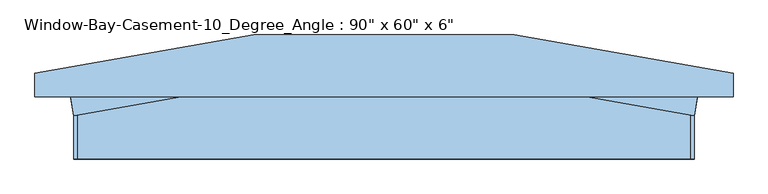
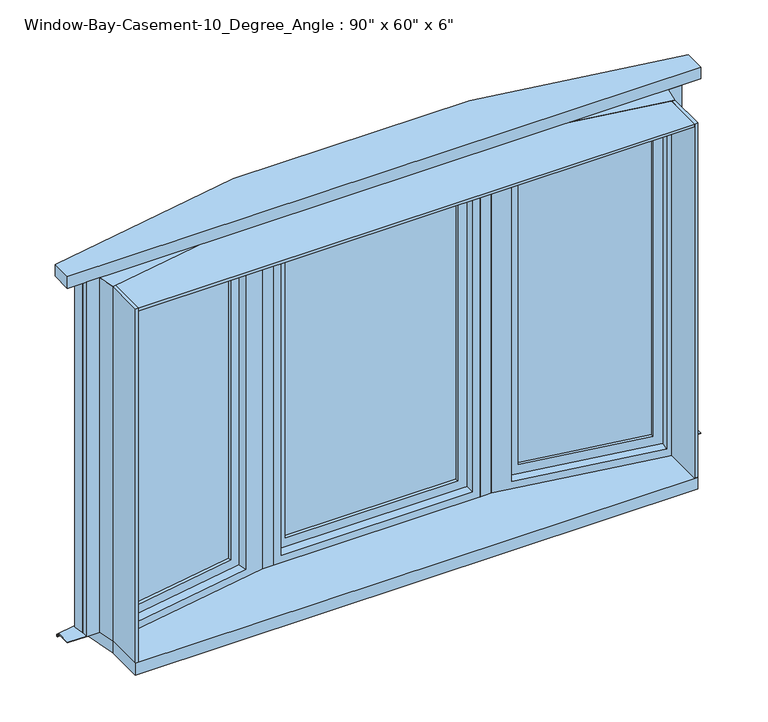
"""IFC4 building model written with IfcOpenShell, lengths in millimetres: window geometry."""

from ifc_helpers import new_model, si_unit, frame, origin, place, context, project, spatial, polyline, outline, extrude, faceted_brep, source, transform, mapped, element, save


def window_bf21e6cb(model_context):
    return source(origin(), model_context, "Body", "SolidModel", [
        extrude(outline(polyline([(1086.3405037, 126.4293252), (1085.2378377, 120.175796), (588.6035631, 207.7458181), (589.7062291, 213.9993474), (1086.3405037, 126.4293252)])), frame((0.0, 0.0, 730.25), z_axis=(0.0, 0.0, 1.0), x_axis=(1.0, 0.0, 0.0)), (0.0, 0.0, 1.0), 1384.3),
        extrude(outline(polyline([(1084.1351718, 113.9222667), (1083.0325059, 107.6687375), (586.3982313, 195.2387597), (587.5008972, 201.4922889), (1084.1351718, 113.9222667)])), frame((0.0, 0.0, 730.25), z_axis=(0.0, 0.0, 1.0), x_axis=(1.0, 0.0, 0.0)), (0.0, 0.0, 1.0), 1384.3),
        extrude(outline(polyline([(1441.45, 57.15), (1441.45, -561.4456588), (-57.15, -561.4456588), (-57.15, 57.15), (1441.45, 57.15)]), holes=[polyline([(1384.3, -504.2956588), (1384.3, 0.0), (0.0, 0.0), (0.0, -504.2956588), (1384.3, -504.2956588)])]), frame((1080.827174, 95.1616791, 730.25), z_axis=(0.17364817766693028, 0.9848077530122081, 0.0), x_axis=(0.0, 0.0, 1.0)), (0.0, 0.0, 1.0), 44.45),
        faceted_brep([(464.7780905, 165.1, 2184.4), (1143.0, 45.5111785, 2184.4), (1155.1293252, 114.3, 2184.4), (1210.6708887, 114.3, 2184.4), (1210.6708887, 136.7463187, 2184.4), (473.6669387, 266.7, 2184.4), (1137.1089371, 85.2376857, 2171.7), (527.9111363, 192.6556946, 2171.7), (538.9377956, 255.1909869, 2171.7), (1148.1355964, 147.772978, 2171.7), (1111.7323538, 51.0245081, 2152.65), (540.0557285, 151.8265214, 2152.65), (546.671724, 189.3476968, 2152.65), (1118.3483494, 88.5456835, 2152.65), (527.9111363, 192.6556946, 673.1), (538.9377956, 255.1909869, 673.1), (540.0557285, 151.8265214, 692.15), (546.671724, 189.3476968, 692.15), (473.6669387, 266.7, 660.4), (1210.6708887, 136.7463187, 660.4), (1210.6708887, 114.3, 660.4), (1155.1293252, 114.3, 660.4), (1143.0, 45.5111785, 660.4), (464.7780905, 165.1, 660.4), (1137.1089371, 85.2376857, 673.1), (1148.1355964, 147.772978, 673.1), (1111.7323538, 51.0245081, 692.15), (1118.3483494, 88.5456835, 692.15)], [[[0, 1, 2, 3, 4, 5]], [[6, 7, 8, 9]], [[10, 11, 12, 13]], [[7, 14, 15, 8]], [[11, 16, 17, 12]], [[18, 19, 20, 21, 22, 23]], [[14, 24, 25, 15]], [[16, 26, 27, 17]], [[22, 21, 2, 1]], [[4, 19, 18, 5], [8, 15, 25, 9]], [[9, 25, 24, 6]], [[6, 24, 14, 7], [12, 17, 27, 13]], [[13, 27, 26, 10]], [[1, 0, 23, 22], [10, 26, 16, 11]], [[5, 18, 23, 0]], [[2, 21, 20, 3]], [[3, 20, 19, 4]]]),
        extrude(outline(polyline([(-1086.3405037, 126.4293252), (-589.7062291, 213.9993474), (-588.6035631, 207.7458181), (-1085.2378377, 120.175796), (-1086.3405037, 126.4293252)])), frame((0.0, 0.0, 730.25), z_axis=(0.0, 0.0, 1.0), x_axis=(1.0, 0.0, 0.0)), (0.0, 0.0, 1.0), 1384.3),
        extrude(outline(polyline([(-1084.1351718, 113.9222667), (-587.5008972, 201.4922889), (-586.3982313, 195.2387597), (-1083.0325059, 107.6687375), (-1084.1351718, 113.9222667)])), frame((0.0, 0.0, 730.25), z_axis=(0.0, 0.0, 1.0), x_axis=(1.0, 0.0, 0.0)), (0.0, 0.0, 1.0), 1384.3),
        extrude(outline(polyline([(1441.45, -57.15), (-57.15, -57.15), (-57.15, 561.4456588), (1441.45, 561.4456588), (1441.45, -57.15)]), holes=[polyline([(1384.3, 504.2956588), (0.0, 504.2956588), (0.0, 0.0), (1384.3, 0.0), (1384.3, 504.2956588)])]), frame((-1080.827174, 95.1616791, 730.25), z_axis=(-0.17364817766693028, 0.9848077530122081, 0.0), x_axis=(0.0, 0.0, 1.0)), (0.0, 0.0, 1.0), 44.45),
        faceted_brep([(-464.7780905, 165.1, 2184.4), (-473.6669387, 266.7, 2184.4), (-1210.6708887, 136.7463187, 2184.4), (-1210.6708887, 114.3, 2184.4), (-1155.1293252, 114.3, 2184.4), (-1143.0, 45.5111785, 2184.4), (-1137.1089371, 85.2376857, 2171.7), (-1148.1355964, 147.772978, 2171.7), (-538.9377956, 255.1909869, 2171.7), (-527.9111363, 192.6556946, 2171.7), (-1111.7323538, 51.0245081, 2152.65), (-1118.3483494, 88.5456835, 2152.65), (-546.671724, 189.3476968, 2152.65), (-540.0557285, 151.8265214, 2152.65), (-538.9377956, 255.1909869, 673.1), (-527.9111363, 192.6556946, 673.1), (-546.671724, 189.3476968, 692.15), (-540.0557285, 151.8265214, 692.15), (-473.6669387, 266.7, 660.4), (-464.7780905, 165.1, 660.4), (-1143.0, 45.5111785, 660.4), (-1155.1293252, 114.3, 660.4), (-1210.6708887, 114.3, 660.4), (-1210.6708887, 136.7463187, 660.4), (-1148.1355964, 147.772978, 673.1), (-1137.1089371, 85.2376857, 673.1), (-1118.3483494, 88.5456835, 692.15), (-1111.7323538, 51.0245081, 692.15)], [[[0, 1, 2, 3, 4, 5]], [[6, 7, 8, 9]], [[10, 11, 12, 13]], [[9, 8, 14, 15]], [[13, 12, 16, 17]], [[18, 19, 20, 21, 22, 23]], [[15, 14, 24, 25]], [[17, 16, 26, 27]], [[20, 5, 4, 21]], [[2, 1, 18, 23], [8, 7, 24, 14]], [[7, 6, 25, 24]], [[6, 9, 15, 25], [12, 11, 26, 16]], [[11, 10, 27, 26]], [[5, 20, 19, 0], [10, 13, 17, 27]], [[1, 0, 19, 18]], [[4, 3, 22, 21]], [[3, 2, 23, 22]]]),
        faceted_brep([(-478.1113628, 317.5, 660.4), (-478.1113628, 317.5, 653.0697935), (478.1113628, 317.5, 653.0697935), (478.1113628, 317.5, 660.4), (-473.6669387, 266.7, 663.1486341), (-473.6669387, 266.7, 660.4), (473.6669387, 266.7, 660.4), (473.6669387, 266.7, 663.1486341), (-478.2335845, 318.897, 654.4483503), (-478.2335845, 318.897, 663.1486341), (478.2335845, 318.897, 663.1486341), (478.2335845, 318.897, 654.4483503), (479.3446905, 331.597, 652.2089977), (-479.3446905, 331.597, 652.2089977), (479.3446905, 331.597, 643.2668038), (-479.3446905, 331.597, 643.2668038), (-478.9980255, 327.6346, 644.7270038), (-478.9980255, 327.6346, 643.2668038), (478.9980255, 327.6346, 643.2668038), (478.9980255, 327.6346, 644.7270038), (-479.2046912, 329.9968, 650.8662705), (-479.2046912, 329.9968, 644.7270038), (479.2046912, 329.9968, 644.7270038), (479.2046912, 329.9968, 650.8662705), (-1286.8726318, 174.8935673, 660.4), (-1286.8726318, 174.8935673, 653.0697935), (1286.8726318, 174.8935673, 660.4), (1286.8726318, 114.3, 660.4), (1210.6726318, 114.3, 660.4), (1210.6726318, 136.7460114, 660.4), (-1210.6726318, 136.7460114, 660.4), (-1210.6726318, 114.3, 660.4), (-1286.8726318, 114.3, 660.4), (-1210.6726318, 136.7460114, 663.1486341), (1210.6726318, 136.7460114, 663.1486341), (1210.6726318, 114.3, 663.1486341), (1286.8726318, 114.3, 663.1486341), (1286.8726318, 176.3121183, 663.1486341), (-1286.8726318, 176.3121183, 663.1486341), (-1286.8726318, 114.3, 663.1486341), (-1210.6726318, 114.3, 663.1486341), (-1286.8726318, 176.3121183, 654.4483503), (-1286.8726318, 189.2080363, 652.2089977), (-1286.8726318, 189.2080363, 643.2668038), (1286.8726318, 189.2080363, 643.2668038), (1286.8726318, 185.1845099, 643.2668038), (-1286.8726318, 185.1845099, 643.2668038), (-1286.8726318, 185.1845099, 644.7270038), (1286.8726318, 185.1845099, 644.7270038), (1286.8726318, 187.5831506, 644.7270038), (-1286.8726318, 187.5831506, 644.7270038), (-1286.8726318, 187.5831506, 650.8662705), (1286.8726318, 174.8935673, 653.0697935), (1286.8726318, 176.3121183, 654.4483503), (1286.8726318, 189.2080363, 652.2089977), (1286.8726318, 187.5831506, 650.8662705)], [[[0, 1, 2, 3]], [[4, 5, 6, 7]], [[8, 9, 10, 11]], [[8, 11, 12, 13]], [[13, 12, 14, 15]], [[16, 17, 18, 19]], [[20, 21, 22, 23]], [[2, 1, 20, 23]], [[1, 0, 24, 25]], [[0, 3, 26, 27, 28, 29, 6, 5, 30, 31, 32, 24]], [[5, 4, 33, 30]], [[4, 7, 34, 35, 36, 37, 10, 9, 38, 39, 40, 33]], [[9, 8, 41, 38]], [[8, 13, 42, 41]], [[13, 15, 43, 42]], [[15, 14, 44, 45, 18, 17, 46, 43]], [[17, 16, 47, 46]], [[16, 19, 48, 49, 22, 21, 50, 47]], [[21, 20, 51, 50]], [[20, 1, 25, 51]], [[3, 2, 52, 26]], [[7, 6, 29, 34]], [[11, 10, 37, 53]], [[12, 11, 53, 54]], [[14, 12, 54, 44]], [[19, 18, 45, 48]], [[23, 22, 49, 55]], [[2, 23, 55, 52]], [[25, 24, 32, 39, 38, 41, 42, 43, 46, 47, 50, 51]], [[27, 26, 52, 55, 49, 48, 45, 44, 54, 53, 37, 36]], [[33, 40, 31, 30]], [[40, 39, 32, 31]], [[36, 35, 28, 27]], [[35, 34, 29, 28]]]),
        extrude(outline(polyline([(-1179.4049856, 142.259341), (-1210.6726318, 136.7460114), (-1218.3912933, 180.520716), (-1187.1236471, 186.0340456), (-1179.4049856, 142.259341)])), frame((0.0, 0.0, 663.1486341), z_axis=(0.0, 0.0, 1.0), x_axis=(1.0, 0.0, 0.0)), (0.0, 0.0, 1.0), 1521.2513659),
        extrude(outline(polyline([(1179.4049856, 142.259341), (1187.1236471, 186.0340456), (1218.3912933, 180.520716), (1210.6726318, 136.7460114), (1179.4049856, 142.259341)])), frame((0.0, 0.0, 663.1486341), z_axis=(0.0, 0.0, 1.0), x_axis=(1.0, 0.0, 0.0)), (0.0, 0.0, 1.0), 1521.2513659),
        extrude(outline(polyline([(480.3335749, 342.9), (1286.8726318, 200.6854033), (1286.8726318, 114.3), (-1286.8708887, 114.3), (-1286.8708887, 200.6857106), (-480.3335749, 342.9), (480.3335749, 342.9)])), frame((0.0, 0.0, 2184.4), z_axis=(0.0, 0.0, 1.0), x_axis=(1.0, 0.0, 0.0)), (0.0, 0.0, 1.0), 50.8),
        extrude(outline(polyline([(-420.0891737, 266.7), (-420.0891737, 165.1), (-464.7780905, 165.1), (-473.6669387, 266.7), (-420.0891737, 266.7)])), frame((0.0, 0.0, 660.4), z_axis=(0.0, 0.0, 1.0), x_axis=(1.0, 0.0, 0.0)), (0.0, 0.0, 1.0), 1524.0),
        extrude(outline(polyline([(473.6669387, 266.7), (464.7780905, 165.1), (420.0891737, 165.1), (420.0891737, 266.7), (473.6669387, 266.7)])), frame((0.0, 0.0, 660.4), z_axis=(0.0, 0.0, 1.0), x_axis=(1.0, 0.0, 0.0)), (0.0, 0.0, 1.0), 1524.0),
        faceted_brep([(407.3891737, 203.2, 673.1), (407.3891737, 266.7, 673.1), (-407.3891737, 266.7, 673.1), (-407.3891737, 203.2, 673.1), (388.3391737, 165.1, 692.15), (388.3391737, 203.2, 692.15), (-388.3391737, 203.2, 692.15), (-388.3391737, 165.1, 692.15), (420.0891737, 266.7, 660.4), (420.0891737, 165.1, 660.4), (-420.0891737, 165.1, 660.4), (-420.0891737, 266.7, 660.4), (-407.3891737, 266.7, 2171.7), (-407.3891737, 203.2, 2171.7), (-388.3391737, 203.2, 2152.65), (-388.3391737, 165.1, 2152.65), (-420.0891737, 165.1, 2184.4), (-420.0891737, 266.7, 2184.4), (407.3891737, 266.7, 2171.7), (407.3891737, 203.2, 2171.7), (388.3391737, 203.2, 2152.65), (388.3391737, 165.1, 2152.65), (420.0891737, 165.1, 2184.4), (420.0891737, 266.7, 2184.4)], [[[0, 1, 2, 3]], [[4, 5, 6, 7]], [[8, 9, 10, 11]], [[3, 2, 12, 13]], [[7, 6, 14, 15]], [[11, 10, 16, 17]], [[13, 12, 18, 19]], [[15, 14, 20, 21]], [[17, 16, 22, 23]], [[11, 17, 23, 8], [1, 18, 12, 2]], [[19, 18, 1, 0]], [[3, 13, 19, 0], [5, 20, 14, 6]], [[21, 20, 5, 4]], [[9, 22, 16, 10], [7, 15, 21, 4]], [[23, 22, 9, 8]]]),
        extrude(outline(polyline([(350.2391737, 234.95), (350.2391737, 228.6), (-350.2391737, 228.6), (-350.2391737, 234.95), (350.2391737, 234.95)])), frame((0.0, 0.0, 730.25), z_axis=(0.0, 0.0, 1.0), x_axis=(1.0, 0.0, 0.0)), (0.0, 0.0, 1.0), 1384.3),
        extrude(outline(polyline([(350.2391737, 222.25), (350.2391737, 215.9), (-350.2391737, 215.9), (-350.2391737, 222.25), (350.2391737, 222.25)])), frame((0.0, 0.0, 730.25), z_axis=(0.0, 0.0, 1.0), x_axis=(1.0, 0.0, 0.0)), (0.0, 0.0, 1.0), 1384.3),
        extrude(outline(polyline([(1143.0, -114.3), (-1143.0, -114.3), (-1143.0, 45.5111785), (-1169.4639823, 195.59588), (-478.1113628, 317.5), (478.1113628, 317.5), (1169.4639823, 195.59588), (1143.0, 45.5111785), (1143.0, -114.3)])), frame((0.0, 0.0, 609.6), z_axis=(0.0, 0.0, 1.0), x_axis=(1.0, 0.0, 0.0)), (0.0, 0.0, 1.0), 50.8),
        extrude(outline(polyline([(2171.7, -407.3891737), (673.1, -407.3891737), (673.1, 407.3891737), (2171.7, 407.3891737), (2171.7, -407.3891737)]), holes=[polyline([(2114.55, 350.2391737), (730.25, 350.2391737), (730.25, -350.2391737), (2114.55, -350.2391737), (2114.55, 350.2391737)])]), frame((0.0, 203.2, 0.0), z_axis=(0.0, 1.0, 0.0), x_axis=(0.0, 0.0, 1.0)), (0.0, 0.0, 1.0), 44.45),
        extrude(outline(polyline([(-1143.0, -114.3), (-1143.0, 45.5111785), (-1130.3, 47.7505311), (-1130.3, -114.3), (-1143.0, -114.3)])), frame((0.0, 0.0, 660.4), z_axis=(0.0, 0.0, 1.0), x_axis=(1.0, 0.0, 0.0)), (0.0, 0.0, 1.0), 1524.0),
        extrude(outline(polyline([(1143.0, -114.3), (1130.3, -114.3), (1130.3, 47.7505311), (1143.0, 45.5111785), (1143.0, -114.3)])), frame((0.0, 0.0, 660.4), z_axis=(0.0, 0.0, 1.0), x_axis=(1.0, 0.0, 0.0)), (0.0, 0.0, 1.0), 1524.0),
        extrude(outline(polyline([(-464.7780905, 165.1), (464.7780905, 165.1), (1130.3, 47.7505311), (1130.3, -114.3), (-1130.3, -114.3), (-1130.3, 47.7505311), (-464.7780905, 165.1)])), frame((0.0, 0.0, 2171.7), z_axis=(0.0, 0.0, 1.0), x_axis=(1.0, 0.0, 0.0)), (0.0, 0.0, 1.0), 12.7),
    ])


if __name__ == "__main__":
    model = new_model("IFC4")
    model_context = context("Model", 3, world=origin())
    ifc_project = project(units=[si_unit("LENGTHUNIT", "METRE", prefix="MILLI")], contexts=[model_context])
    site = spatial("IfcSite", under=ifc_project)
    building = spatial("IfcBuilding", under=site)
    placement = place(None, origin())
    window_shape = window_bf21e6cb(model_context)
    element("IfcWindow", 1, ObjectType="Window-Bay-Casement-10_Degree_Angle : 90\" x 60\" x 6\"", at=placement, inside=building, context=model_context, shape_type="MappedRepresentation", body=[
        mapped(window_shape, transform((0.0, 0.0, 0.0), x_axis=(1.0, 0.0, 0.0), y_axis=(0.0, 1.0, 0.0), z_axis=(0.0, 0.0, 1.0))),
    ])
    save(model, "model.ifc")

# Revit data of these elements
# Type "Window-Bay-Casement-10_Degree_Angle : 90\" x 60\" x 6\""
#   Type Mark = "21"
#   Fire Rating = "0.5h"
#   Assembly Code = "B2020100"
#   Analytic Construction = "Double glazing - domestic"
#   Width of Middle Sash = 2' - 9.07789"
#   Width = 7' - 6"
#   Visual Light Transmittance = 0.81
#   Thermal Resistance (R) = 1.8146 (h·ft²·°F)/BTU
#   Solar Heat Gain Coefficient = 0.76
#   Rough Width = 7' - 6 1/2"
#   Rough Height = 5' - 0 1/2"
#   Length 4 = 0' - 0.24059"
#   Length 3 = 0' - 0 7/64"
#   Length 2 = 3' - 1.29661"
#   Length 1 = 2' - 2.46106"
#   Wall Thickness [instance default] = 0' - 6"
#   Trim Width = 7' - 10.21872"
#   Trim Height = 5' - 0"
#   Height 1 = 5' - 2"
#   Height = 5' - 0"
#   Heat Transfer Coefficient (U) = 0.5511 BTU/(h·ft²·°F)
#   Depth = 0' - 6"
#   Default Sill Height = 2' - 0"
#   Angle 1 = 5.00°
#   Angle = 10.00°
#   Center Muntin Visibility = yes
#   Side Muntin Visibility = yes
#   Interior Trim Visibility [instance default] = yes
#   Exterior Trim Visibility [instance default] = yes
#   Center Muntin Pattern = Muntin Pattern_2x2 : Muntin Pattern_2x2
#   Side Muntin Pattern = Muntin Pattern_2x2 : Muntin Pattern_2x2
#   Interior Trim Material = Wood - Stained
#   Exterior Trim Material = Clad - White
#   Exterior Trim = element 436057
#   Interior Trim = Trim-Window-Interior-Flat : Picture Frame
#   Interior Frame Material = Wood - Stained
#   Glass Panel Material = Glass
#   Exterior Frame Material = Clad - White
#   Wall Closure = (empty or 0)
# Element 1 (IfcWindow, "Window-Bay-Casement-10_Degree_Angle : 90\" x 60\" x 6\"")
#   Wall Thickness = 0' - 9"
#   Materials on its faces: "Clad - White", "Wood - Stained", "Glass"
# Materials
#   "Wood - Stained": class "Wood", colour RGB 224 178 126, transparency 0, Cost = 0
#   "Clad - White": class "Wood", colour RGB 242 242 238, transparency 0, Cost = 0
#   "Glass": class "Glass", colour RGB 0 128 192, transparency 0.75, Description = "Soda Lime Glass", Cost = 0
